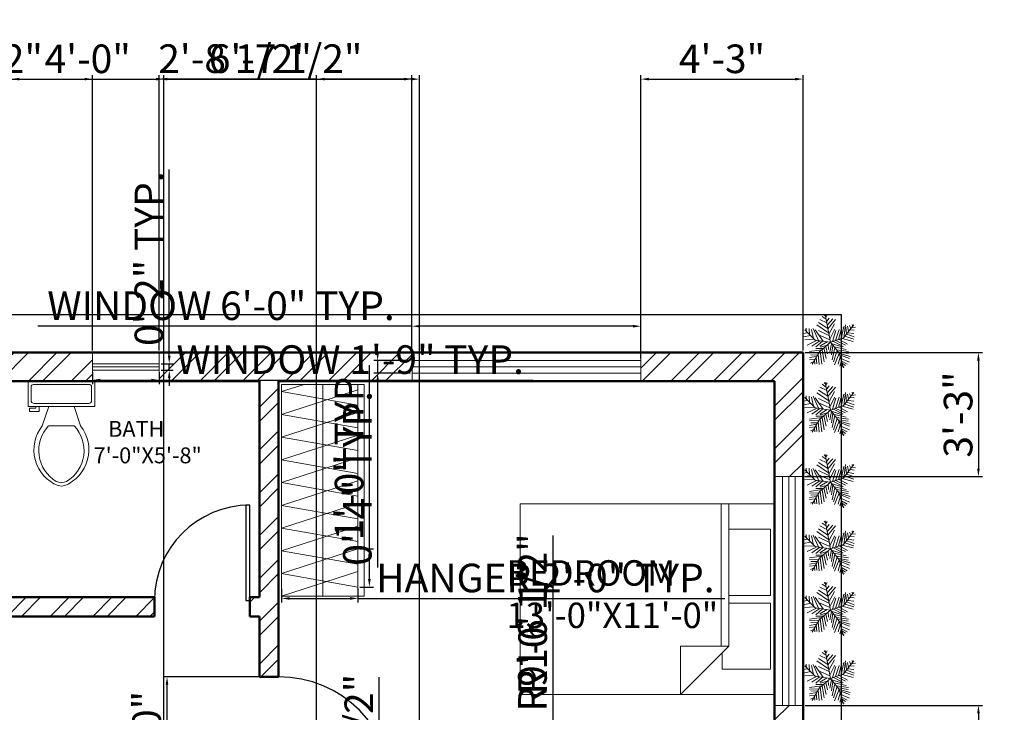
# Model space of a CAD drawing. Units: inches. Extents: x 176 to 806, y 915 to 1663.
# Tile 5 of 5: x 482 to 792, y 1445 to 1663. Entities that reach past the tile are written whole.
import ezdxf

# ---------------------------------------------------------------- set-up
doc = ezdxf.new("R2010")
doc.units = ezdxf.units.IN
for name, color, linetype, lineweight in [('A-ANNO-DIMS', 2, 'Continuous', 18), ('A-AREA-IDEN', 7, 'Continuous', 18), ('A-DOOR', 4, 'Continuous', 25), ('A-FLOR-CASE', 8, 'Continuous', 18), ('A-FLOR-FIXT', 9, 'Continuous', 18), ('A-FURN', 8, 'Continuous', 18), ('A-WALL', 7, 'Continuous', 50), ('A-WALL-PATT', 252, 'Continuous', 13), ('C-PROP', 8, 'Continuous', 25), ('L-PLNT', 3, 'Continuous', 13)]:
    doc.layers.add(name, color=color, linetype=linetype, lineweight=lineweight)
doc.layers.add('A-GLAZ', color=244, linetype='Continuous', lineweight=18, true_color=0x991b1e)
doc.styles.get("Standard").update_dxf_attribs({"font": 'arial.ttf'})
doc.dimstyles.new('ISO-25', dxfattribs={"dimtxt": 9, "dimasz": 2.5, "dimexe": 1.25, "dimexo": 0.625, "dimtad": 1, "dimlunit": 3, "dimtxsty": 'Standard', "dimcen": 2.5, "dimadec": 0, "dimazin": 0, "dimtfac": 1, "dimtmove": 0, "dimatfit": 3, "dimfxl": 1, "dimarcsym": 0})

# ---------------------------------------------------------------- blocks, each defined once
blk = doc.blocks.new('*U3')
for p, q in [((0, 0), (0, -6)), ((-40, 0), (-40, -6))]:
    blk.add_line(p, q)
blk.add_lwpolyline([(0, 0), (0, 40), (-1.75, 40), (-1.75, 0)], close=True)
blk.add_arc((0, 0), 40, 90, 180)
blk = doc.blocks.new('*U8')
for p, q in [((-5.114, 28.097), (-24.676, 40.636)), ((-7.288, 39.707), (-21.778, 46.673)), ((-8.737, 47.138), (-17.069, 52.711)), ((-10.186, 53.64), (-13.084, 55.962)), ((0, 0), (-10.5, 57)), ((-9.099, 51.782), (-6.563, 55.962)), ((-7.65, 43.423), (-2.578, 49.46)), ((-5.839, 35.992), (4.667, 48.067)), ((-5.114, 27.632), (10.463, 46.673)), ((-31.5, 4.5), (-52.5, 25.5)), ((-48.585, 21.131), (-49.309, 29.026)), ((-43.513, 28.561), (-42.427, 15.558)), ((-38.442, 26.239), (-34.819, 7.663)), ((-35.544, 28.097), (-24.314, 3.947)), ((-14.533, 2.09), (-30.834, 25.31)), ((-3.665, 19.273), (-27.574, 35.527)), ((-24.314, 23.917), (-2.941, 13.7)), ((-2.941, 16.486), (8.652, 37.85)), ((-1.129, 6.734), (9.014, 26.704)), ((3.942, 1.625), (11.187, 24.381)), ((10.101, 3.483), (17.708, 26.239)), ((16.259, 5.805), (23.142, 31.348)), ((22.055, 7.198), (27.489, 32.277)), ((27, 9), (48, 36)), ((27.127, 9.056), (31.112, 35.992)), ((31.836, 30.883), (32.561, 16.486)), ((35.096, 32.741), (37.27, 22.524)), ((38.719, 34.134), (41.979, 28.561)), ((40.53, 25.775), (48.862, 24.846)), ((43.791, 29.954), (51.036, 30.883)), ((44.153, 36.456), (45.239, 32.741)), ((-47.498, 19.737), (-55.83, 18.344)), ((-40.615, 13.7), (-55.105, 10.913)), ((-33.37, 6.269), (-52.207, 5.34)), ((-28.299, 3.483), (-47.86, -5.805)), ((-21.416, 3.018), (-38.079, -8.128)), ((0, 0), (-31.5, 4.5)), ((-15.982, 2.09), (-30.11, -9.521)), ((0, 0), (-22.5, -19.5)), ((-6.563, 1.161), (-21.416, -8.128)), ((-20.691, 13.7), (-1.129, 4.876)), ((0, 0), (27, 9)), ((0, 0), (18, -22.5)), ((6.478, 1.625), (26.04, -8.592)), ((11.187, 3.483), (30.749, -5.805)), ((18.07, 5.805), (35.096, -3.483)), ((24.229, 7.663), (46.688, 1.625)), ((29.662, 12.307), (48.137, 6.269)), ((33.285, 16.486), (48.862, 10.913)), ((36.183, 19.737), (48.137, 17.88)), ((-17.431, -15.094), (-42.789, -18.809)), ((-22.5, -19.5), (-37.5, -45)), ((-15.257, -12.772), (-30.11, -12.772)), ((-20.691, -18.345), (-17.793, -44.352)), ((-6.563, -5.805), (-19.967, -9.985)), ((-17.069, -15.094), (-12.721, -40.172)), ((-13.446, -11.378), (-8.737, -32.741)), ((-9.461, -8.592), (-6.201, -23.453)), ((-4.752, -3.483), (-3.665, -14.629)), ((2.493, -3.019), (-1.491, -20.202)), ((1.769, -2.555), (24.229, -9.521)), ((5.029, -6.27), (2.131, -25.775)), ((9.014, -11.378), (3.58, -35.992)), ((14.085, -16.951), (6.478, -40.172)), ((7.565, -9.056), (32.198, -14.629)), ((12.274, -15.094), (36.907, -18.809)), ((16.259, -19.738), (36.183, -22.989)), ((-28.299, -29.026), (-42.789, -31.348)), ((-24.314, -21.596), (-42.427, -22.06)), ((-30.834, -34.135), (-42.427, -35.528)), ((-34.457, -39.708), (-40.978, -42.494)), ((-26.849, -26.24), (-40.253, -25.775)), ((-32.646, -36.921), (-31.921, -44.352)), ((-29.023, -30.884), (-27.936, -43.887)), ((-25.038, -23.918), (-22.865, -45.281)), ((18.07, -22.524), (8.289, -45.745)), ((20.244, -30.419), (15.897, -44.816)), ((18, -22.5), (27, -52.5)), ((18.433, -22.524), (40.53, -29.026)), ((19.157, -25.311), (38.719, -33.206)), ((22.78, -37.85), (19.519, -48.532)), ((21.331, -32.741), (39.081, -40.636)), ((22.78, -38.314), (34.372, -44.816)), ((24.591, -45.745), (23.142, -50.854)), ((24.591, -43.423), (30.749, -47.603)), ((26.764, -49.925), (28.213, -50.854))]:
    blk.add_line(p, q)
blk = doc.blocks.new('Bed - Queen')
for p, q in [((0, -80.00003), (0, 0)), ((0, 0), (59.99999, 0)), ((59.99999, 0), (59.99999, -80.00003)), ((7.99999, -1.2), (28.79998, -1.2)), ((7.99999, -14.4), (7.99999, -1.2)), ((28.79998, -1.2), (28.79998, -14.4)), ((31.19999, -1.2), (51.99999, -1.2)), ((31.19999, -14.4), (31.19999, -1.2)), ((51.99999, -1.2), (51.99999, -16.4)), ((0, -14.4), (44.8, -14.4)), ((59.99999, -29.6), (44.8, -14.4)), ((44.8, -14.4), (44.8, -29.6)), ((44.8, -16.8), (0, -16.8)), ((51.99999, -16.4), (46.79936, -16.4)), ((44.8, -29.6), (59.99999, -29.6)), ((59.99999, -80.00003), (0, -80.00003))]:
    blk.add_line(p, q)
blk = doc.blocks.new('*U13')
for p, q in [((9.5, -6), (9.5, -2)), ((-10, -8.5), (-8, -8.5)), ((-10, -9.5), (-10, -8.5)), ((-8, -8.5), (-8, -8)), ((-7, -8), (-7, -9.5)), ((-4, -8), (-6, -14)), ((4, -8), (6, -14)), ((-7, -9.5), (-10, -9.5)), ((4, -14), (-4, -14))]:
    blk.add_line(p, q)
blk.add_lwpolyline([(10.5, -8), (10.5, 0), (-10.5, 0), (-10.5, -8)], close=True)
for points in [[(-9.5, -2), (-9.5, -6)], [(8.5, -1), (-8.5, -1)], [(-8.5, -7), (8.5, -7)]]:
    blk.add_lwpolyline(points)
for centre, radius, start, end in [((-8.62, -1.88), 0.884, 81.8699, 188.1301), ((8.62, -1.88), 0.884, 351.8699, 98.1301), ((-8.62, -6.12), 0.884, 171.8699, 278.1301), ((8.62, -6.12), 0.884, 261.8699, 8.1301), ((3.52, -21.58), 12.17, 141.4691, 247.9714), ((4.2, -21.82), 11.33, 136.3677, 238.9468), ((-3.52, -21.58), 12.17, 292.0284, 38.5307), ((-4.2, -21.82), 11.33, 301.053, 43.6321), ((0, -27.88), 4, 245.7318, 294.2682), ((0, -29), 4, 254.8605, 285.1395)]:
    blk.add_arc(centre, radius, start, end)
blk = doc.blocks.new('WIN-GLAZING-72IN')
for p, q in [((0, 2), (72, 2)), ((0, 0), (72, 0)), ((0, -2), (72, -2))]:
    blk.add_line(p, q)
blk = doc.blocks.new('WIN-GLAZING-21IN')
for p, q in [((0, 1), (21, 1)), ((0, 0), (21, 0)), ((0, -1), (21, -1))]:
    blk.add_line(p, q)
blk = doc.blocks.new('WARDROBE-HANGER')
for p, q in [((0, 0), (24, 7.76)), ((24, -4.24), (0, 0))]:
    blk.add_line(p, q)
blk = doc.blocks.new('*D22')
at = {"layer": 'A-ANNO-DIMS', "color": 0, "lineweight": -2, "transparency": 16777216}
for p, q in [((564.7, 1483.83), (564.7, 1479.6)), ((588.7, 1483.83), (588.7, 1479.6)), ((567.2, 1480.85), (586.2, 1480.85)), ((588.7, 1480.85), (704.11, 1480.85))]:
    blk.add_line(p, q, dxfattribs=at)
at = {"layer": 'A-ANNO-DIMS', "color": 0, "transparency": 16777216}
for points in [[(567.2, 1481.27), (567.2, 1480.44), (564.7, 1480.85)], [(586.2, 1481.27), (586.2, 1480.44), (588.7, 1480.85)]]:
    blk.add_solid(points, dxfattribs=at)
at = {"layer": 'Defpoints', "color": 0, "transparency": 16777216}
for p in [(564.7, 1484.45), (588.7, 1484.45), (588.7, 1480.85)]:
    blk.add_point(p, dxfattribs=at)
at = {"layer": 'A-ANNO-DIMS', "color": 0, "transparency": 16777216, "insert": (647.66, 1486.13), "char_height": 9, "attachment_point": 5}
blk.add_mtext('HANGER 2\'-0" TYP.', dxfattribs=at)
blk = doc.blocks.new('*D23')
at = {"layer": 'A-ANNO-DIMS', "color": 0, "lineweight": -2, "transparency": 16777216}
for p, q in [((592.3, 1496.45), (592.3, 1554.21)), ((589.33, 1496.45), (593.55, 1496.45)), ((592.3, 1486.95), (592.3, 1493.95)), ((589.33, 1484.45), (593.55, 1484.45))]:
    blk.add_line(p, q, dxfattribs=at)
at = {"layer": 'A-ANNO-DIMS', "color": 0, "transparency": 16777216}
for points in [[(591.89, 1493.95), (592.72, 1493.95), (592.3, 1496.45)], [(591.89, 1486.95), (592.72, 1486.95), (592.3, 1484.45)]]:
    blk.add_solid(points, dxfattribs=at)
at = {"layer": 'Defpoints', "color": 0, "transparency": 16777216}
for p in [(588.7, 1496.45), (592.3, 1496.45), (588.7, 1484.45)]:
    blk.add_point(p, dxfattribs=at)
at = {"layer": 'A-ANNO-DIMS', "color": 0, "transparency": 16777216, "insert": (587.08, 1526.58), "char_height": 9, "attachment_point": 5, "rotation": 90}
blk.add_mtext('1\'-0" TYP.', dxfattribs=at)
blk = doc.blocks.new('*D24')
at = {"layer": 'A-ANNO-DIMS', "color": 0, "lineweight": -2, "transparency": 16777216}
for p, q in [((605.7, 1556.33), (605.7, 1567.76)), ((677.7, 1556.33), (677.7, 1567.76)), ((605.7, 1566.51), (488.07, 1566.51)), ((675.2, 1566.51), (608.2, 1566.51))]:
    blk.add_line(p, q, dxfattribs=at)
at = {"layer": 'A-ANNO-DIMS', "color": 0, "transparency": 16777216}
for points in [[(608.2, 1566.92), (608.2, 1566.09), (605.7, 1566.51)], [(675.2, 1566.92), (675.2, 1566.09), (677.7, 1566.51)]]:
    blk.add_solid(points, dxfattribs=at)
at = {"layer": 'Defpoints', "color": 0, "transparency": 16777216}
for p in [(605.7, 1566.51), (605.7, 1555.71), (677.7, 1555.71)]:
    blk.add_point(p, dxfattribs=at)
at = {"layer": 'A-ANNO-DIMS', "color": 0, "transparency": 16777216, "insert": (545.64, 1571.79), "char_height": 9, "attachment_point": 5}
blk.add_mtext('WINDOW 6\'-0" TYP.', dxfattribs=at)
blk = doc.blocks.new('*D25')
at = {"layer": 'A-ANNO-DIMS', "color": 0, "lineweight": -2, "transparency": 16777216}
for p, q in [((594.9, 1558.21), (594.9, 1560.71)), ((605.08, 1555.71), (593.65, 1555.71)), ((594.9, 1555.71), (594.9, 1551.71)), ((605.08, 1551.71), (593.65, 1551.71)), ((594.9, 1549.21), (594.9, 1490.6))]:
    blk.add_line(p, q, dxfattribs=at)
at = {"layer": 'A-ANNO-DIMS', "color": 0, "transparency": 16777216}
for points in [[(594.49, 1558.21), (595.32, 1558.21), (594.9, 1555.71)], [(594.49, 1549.21), (595.32, 1549.21), (594.9, 1551.71)]]:
    blk.add_solid(points, dxfattribs=at)
at = {"layer": 'Defpoints', "color": 0, "transparency": 16777216}
for p in [(605.7, 1555.71), (594.9, 1551.71), (605.7, 1551.71)]:
    blk.add_point(p, dxfattribs=at)
at = {"layer": 'A-ANNO-DIMS', "color": 0, "transparency": 16777216, "insert": (589.68, 1518.65), "char_height": 9, "attachment_point": 5, "rotation": 90}
blk.add_mtext('0\'-4" TYP.', dxfattribs=at)
blk = doc.blocks.new('*D26')
at = {"layer": 'A-ANNO-DIMS', "color": 0, "lineweight": -2, "transparency": 16777216}
for p, q in [((505.2, 1552.08), (505.2, 1548.31)), ((526.2, 1552.08), (526.2, 1548.31)), ((507.7, 1549.56), (523.7, 1549.56)), ((526.2, 1549.56), (643.84, 1549.56))]:
    blk.add_line(p, q, dxfattribs=at)
at = {"layer": 'A-ANNO-DIMS', "color": 0, "transparency": 16777216}
for points in [[(507.7, 1549.97), (507.7, 1549.14), (505.2, 1549.56)], [(523.7, 1549.97), (523.7, 1549.14), (526.2, 1549.56)]]:
    blk.add_solid(points, dxfattribs=at)
at = {"layer": 'Defpoints', "color": 0, "transparency": 16777216}
for p in [(505.2, 1552.71), (526.2, 1552.71), (526.2, 1549.56)]:
    blk.add_point(p, dxfattribs=at)
at = {"layer": 'A-ANNO-DIMS', "color": 0, "transparency": 16777216, "insert": (586.27, 1554.84), "char_height": 9, "attachment_point": 5}
blk.add_mtext('WINDOW 1\'-9" TYP.', dxfattribs=at)
blk = doc.blocks.new('*D27')
at = {"layer": 'A-ANNO-DIMS', "color": 0, "lineweight": -2, "transparency": 16777216}
for p, q in [((529.35, 1557.21), (529.35, 1615.82)), ((526.83, 1554.71), (530.6, 1554.71)), ((529.35, 1552.71), (529.35, 1554.71)), ((526.83, 1552.71), (530.6, 1552.71)), ((529.35, 1550.21), (529.35, 1547.71))]:
    blk.add_line(p, q, dxfattribs=at)
at = {"layer": 'A-ANNO-DIMS', "color": 0, "transparency": 16777216}
for points in [[(528.94, 1557.21), (529.77, 1557.21), (529.35, 1554.71)], [(528.94, 1550.21), (529.77, 1550.21), (529.35, 1552.71)]]:
    blk.add_solid(points, dxfattribs=at)
at = {"layer": 'Defpoints', "color": 0, "transparency": 16777216}
for p in [(526.2, 1554.71), (529.35, 1554.71), (526.2, 1552.71)]:
    blk.add_point(p, dxfattribs=at)
at = {"layer": 'A-ANNO-DIMS', "color": 0, "transparency": 16777216, "insert": (524.13, 1587.76), "char_height": 9, "attachment_point": 5, "rotation": 90}
blk.add_mtext('0\'-2" TYP.', dxfattribs=at)
blk = doc.blocks.new('*D37')
at = {"layer": 'A-ANNO-DIMS', "color": 0, "lineweight": -2, "transparency": 16777216}
for p, q in [((595.42, 1407.41), (595.42, 1456.05)), ((607.4, 1407.41), (594.17, 1407.41)), ((595.42, 1373.24), (595.42, 1404.91)), ((607.4, 1370.74), (594.17, 1370.74))]:
    blk.add_line(p, q, dxfattribs=at)
at = {"layer": 'A-ANNO-DIMS', "color": 0, "transparency": 16777216}
for points in [[(595.01, 1404.91), (595.84, 1404.91), (595.42, 1407.41)], [(595.01, 1373.24), (595.84, 1373.24), (595.42, 1370.74)]]:
    blk.add_solid(points, dxfattribs=at)
at = {"layer": 'Defpoints', "color": 0, "transparency": 16777216}
for p in [(595.42, 1407.41), (608.02, 1407.41), (608.02, 1370.74)]:
    blk.add_point(p, dxfattribs=at)
at = {"layer": 'A-ANNO-DIMS', "color": 0, "transparency": 16777216, "insert": (590.14, 1432.98), "char_height": 9, "attachment_point": 5, "rotation": 90}
blk.add_mtext('3\'-0 1/2"', dxfattribs=at)
blk = doc.blocks.new('*D41')
at = {"layer": 'A-ANNO-DIMS', "color": 0, "lineweight": -2, "transparency": 16777216}
for p, q in [((425.7, 1558.83), (425.7, 1645.51)), ((505.2, 1558.83), (505.2, 1645.51)), ((428.2, 1644.26), (502.7, 1644.26))]:
    blk.add_line(p, q, dxfattribs=at)
at = {"layer": 'A-ANNO-DIMS', "color": 0, "transparency": 16777216}
for points in [[(428.2, 1644.67), (428.2, 1643.84), (425.7, 1644.26)], [(502.7, 1644.67), (502.7, 1643.84), (505.2, 1644.26)]]:
    blk.add_solid(points, dxfattribs=at)
at = {"layer": 'Defpoints', "color": 0, "transparency": 16777216}
for p in [(505.2, 1644.26), (425.7, 1558.21), (505.2, 1558.21)]:
    blk.add_point(p, dxfattribs=at)
at = {"layer": 'A-ANNO-DIMS', "color": 0, "transparency": 16777216, "insert": (465.45, 1649.53), "char_height": 9, "attachment_point": 5}
blk.add_mtext('6\'-7 1/2"', dxfattribs=at)
blk = doc.blocks.new('*D42')
at = {"layer": 'A-ANNO-DIMS', "color": 0, "lineweight": -2, "transparency": 16777216}
for p, q in [((526.2, 1558.83), (526.2, 1645.51)), ((605.7, 1558.83), (605.7, 1645.51)), ((528.7, 1644.26), (603.2, 1644.26))]:
    blk.add_line(p, q, dxfattribs=at)
at = {"layer": 'A-ANNO-DIMS', "color": 0, "transparency": 16777216}
for points in [[(528.7, 1644.67), (528.7, 1643.84), (526.2, 1644.26)], [(603.2, 1644.67), (603.2, 1643.84), (605.7, 1644.26)]]:
    blk.add_solid(points, dxfattribs=at)
at = {"layer": 'Defpoints', "color": 0, "transparency": 16777216}
for p in [(605.7, 1644.26), (526.2, 1558.21), (605.7, 1558.21)]:
    blk.add_point(p, dxfattribs=at)
at = {"layer": 'A-ANNO-DIMS', "color": 0, "transparency": 16777216, "insert": (565.95, 1649.53), "char_height": 9, "attachment_point": 5}
blk.add_mtext('6\'-7 1/2"', dxfattribs=at)
blk = doc.blocks.new('*D43')
at = {"layer": 'A-ANNO-DIMS', "color": 0, "lineweight": -2, "transparency": 16777216}
for p, q in [((677.7, 1558.83), (677.7, 1645.51)), ((728.7, 1558.83), (728.7, 1645.51)), ((680.2, 1644.26), (726.2, 1644.26))]:
    blk.add_line(p, q, dxfattribs=at)
at = {"layer": 'A-ANNO-DIMS', "color": 0, "transparency": 16777216}
for points in [[(680.2, 1644.67), (680.2, 1643.84), (677.7, 1644.26)], [(726.2, 1644.67), (726.2, 1643.84), (728.7, 1644.26)]]:
    blk.add_solid(points, dxfattribs=at)
at = {"layer": 'Defpoints', "color": 0, "transparency": 16777216}
for p in [(728.7, 1644.26), (677.7, 1558.21), (728.7, 1558.21)]:
    blk.add_point(p, dxfattribs=at)
at = {"layer": 'A-ANNO-DIMS', "color": 0, "transparency": 16777216, "insert": (703.2, 1649.48), "char_height": 9, "attachment_point": 5}
blk.add_mtext('4\'-3"', dxfattribs=at)
blk = doc.blocks.new('*D44')
at = {"layer": 'A-ANNO-DIMS', "color": 0, "lineweight": -2, "transparency": 16777216}
for p, q in [((729.33, 1558.21), (785.1, 1558.21)), ((783.85, 1555.71), (783.85, 1521.71)), ((729.33, 1519.21), (785.1, 1519.21))]:
    blk.add_line(p, q, dxfattribs=at)
at = {"layer": 'A-ANNO-DIMS', "color": 0, "transparency": 16777216}
for points in [[(783.43, 1555.71), (784.27, 1555.71), (783.85, 1558.21)], [(783.43, 1521.71), (784.27, 1521.71), (783.85, 1519.21)]]:
    blk.add_solid(points, dxfattribs=at)
at = {"layer": 'Defpoints', "color": 0, "transparency": 16777216}
for p in [(728.7, 1558.21), (728.7, 1519.21), (783.85, 1519.21)]:
    blk.add_point(p, dxfattribs=at)
at = {"layer": 'A-ANNO-DIMS', "color": 0, "transparency": 16777216, "insert": (778.63, 1538.71), "char_height": 9, "attachment_point": 5, "rotation": 90}
blk.add_mtext('3\'-3"', dxfattribs=at)
blk = doc.blocks.new('*D45')
at = {"layer": 'A-ANNO-DIMS', "color": 0, "lineweight": -2, "transparency": 16777216}
for p, q in [((729.33, 1447.21), (785.1, 1447.21)), ((783.85, 1444.71), (783.85, 1382.17)), ((729.33, 1379.67), (785.1, 1379.67))]:
    blk.add_line(p, q, dxfattribs=at)
at = {"layer": 'A-ANNO-DIMS', "color": 0, "transparency": 16777216}
for points in [[(783.43, 1444.71), (784.27, 1444.71), (783.85, 1447.21)], [(783.43, 1382.17), (784.27, 1382.17), (783.85, 1379.67)]]:
    blk.add_solid(points, dxfattribs=at)
at = {"layer": 'Defpoints', "color": 0, "transparency": 16777216}
for p in [(728.7, 1447.21), (728.7, 1379.67), (783.85, 1379.67)]:
    blk.add_point(p, dxfattribs=at)
at = {"layer": 'A-ANNO-DIMS', "color": 0, "transparency": 16777216, "insert": (778.57, 1413.44), "char_height": 9, "attachment_point": 5, "rotation": 90}
blk.add_mtext('5\'-7 1/2"', dxfattribs=at)
blk = doc.blocks.new('*D52')
at = {"layer": 'A-ANNO-DIMS', "color": 0, "lineweight": -2, "transparency": 16777216}
for p, q in [((479.7, 1200.83), (479.7, 1645.51)), ((527.7, 1200.83), (527.7, 1645.51)), ((482.2, 1644.26), (525.2, 1644.26))]:
    blk.add_line(p, q, dxfattribs=at)
at = {"layer": 'A-ANNO-DIMS', "color": 0, "transparency": 16777216}
for points in [[(482.2, 1644.67), (482.2, 1643.84), (479.7, 1644.26)], [(525.2, 1644.67), (525.2, 1643.84), (527.7, 1644.26)]]:
    blk.add_solid(points, dxfattribs=at)
at = {"layer": 'Defpoints', "color": 0, "transparency": 16777216}
for p in [(527.7, 1644.26), (479.7, 1200.21), (527.7, 1200.21)]:
    blk.add_point(p, dxfattribs=at)
at = {"layer": 'A-ANNO-DIMS', "color": 0, "transparency": 16777216, "insert": (503.7, 1649.48), "char_height": 9, "attachment_point": 5}
blk.add_mtext('4\'-0"', dxfattribs=at)
blk = doc.blocks.new('*D64')
at = {"layer": 'A-ANNO-DIMS', "color": 0, "lineweight": -2, "transparency": 16777216}
for p, q in [((563.08, 1456.21), (527.4, 1456.21)), ((528.65, 1422.71), (528.65, 1453.71)), ((563.08, 1420.21), (527.4, 1420.21))]:
    blk.add_line(p, q, dxfattribs=at)
at = {"layer": 'A-ANNO-DIMS', "color": 0, "transparency": 16777216}
for points in [[(528.24, 1453.71), (529.07, 1453.71), (528.65, 1456.21)], [(528.24, 1422.71), (529.07, 1422.71), (528.65, 1420.21)]]:
    blk.add_solid(points, dxfattribs=at)
at = {"layer": 'Defpoints', "color": 0, "transparency": 16777216}
for p in [(528.65, 1456.21), (563.7, 1456.21), (563.7, 1420.21)]:
    blk.add_point(p, dxfattribs=at)
at = {"layer": 'A-ANNO-DIMS', "color": 0, "transparency": 16777216, "insert": (523.43, 1438.21), "char_height": 9, "attachment_point": 5, "rotation": 90}
blk.add_mtext('3\'-0"', dxfattribs=at)
blk = doc.blocks.new('*D65')
at = {"layer": 'A-ANNO-DIMS', "color": 0, "lineweight": -2, "transparency": 16777216}
for p, q in [((575.7, 1278.83), (575.7, 1645.51)), ((608.02, 1371.37), (608.02, 1645.51)), ((575.7, 1644.26), (526.9, 1644.26)), ((605.52, 1644.26), (578.2, 1644.26))]:
    blk.add_line(p, q, dxfattribs=at)
at = {"layer": 'A-ANNO-DIMS', "color": 0, "transparency": 16777216}
for points in [[(578.2, 1644.67), (578.2, 1643.84), (575.7, 1644.26)], [(605.52, 1644.67), (605.52, 1643.84), (608.02, 1644.26)]]:
    blk.add_solid(points, dxfattribs=at)
at = {"layer": 'Defpoints', "color": 0, "transparency": 16777216}
for p in [(575.7, 1644.26), (608.02, 1370.74), (575.7, 1278.21)]:
    blk.add_point(p, dxfattribs=at)
at = {"layer": 'A-ANNO-DIMS', "color": 0, "transparency": 16777216, "insert": (550.05, 1649.53), "char_height": 9, "attachment_point": 5}
blk.add_mtext('2\'-8 1/2"', dxfattribs=at)
blk = doc.blocks.new('*D74')
at = {"layer": 'A-ANNO-DIMS', "color": 0, "lineweight": -2, "transparency": 16777216}
for p, q in [((650.03, 1491.85), (650.02, 1401.24)), ((650.02, 1277.55), (650.02, 1398.74))]:
    blk.add_line(p, q, dxfattribs=at)
at = {"layer": 'A-ANNO-DIMS', "color": 0, "transparency": 16777216}
blk.add_solid([(649.61, 1401.24), (650.44, 1401.24), (650.02, 1398.74)], dxfattribs=at)
at = {"layer": 'Defpoints', "color": 0, "transparency": 16777216}
for p in [(650.02, 1398.74), (650.02, 1277.55)]:
    blk.add_point(p, dxfattribs=at)
at = {"layer": 'A-ANNO-DIMS', "color": 0, "transparency": 16777216, "insert": (644.81, 1471.46), "char_height": 9, "attachment_point": 5, "rotation": 89.9999}
blk.add_mtext('R10\'-1"', dxfattribs=at)
blk = doc.blocks.new('*D75')
at = {"layer": 'A-ANNO-DIMS', "color": 0, "lineweight": -2, "transparency": 16777216}
for p, q in [((650.03, 1500.67), (650.02, 1407.24)), ((650.02, 1290.49), (650.02, 1404.74))]:
    blk.add_line(p, q, dxfattribs=at)
at = {"layer": 'A-ANNO-DIMS', "color": 0, "transparency": 16777216}
blk.add_solid([(649.61, 1407.24), (650.44, 1407.24), (650.02, 1404.74)], dxfattribs=at)
at = {"layer": 'Defpoints', "color": 0, "transparency": 16777216}
for p in [(650.02, 1404.74), (650.02, 1290.49)]:
    blk.add_point(p, dxfattribs=at)
at = {"layer": 'A-ANNO-DIMS', "color": 0, "transparency": 16777216, "insert": (644.75, 1473.29), "char_height": 9, "attachment_point": 5, "rotation": 89.9998}
blk.add_mtext('R9\'-6 1/2"', dxfattribs=at)

msp = doc.modelspace()

# ---------------------------------------------------------------- hatches: boundary and pattern name
at = {"layer": 'A-WALL-PATT'}
h = msp.add_hatch(dxfattribs=at)
h.set_pattern_fill('ANSI32', color=256)
h.paths.add_polyline_path([(302.704, 1050.206), (353.704, 1050.206), (353.704, 1059.206), (311.704, 1059.206), (311.704, 1191.206), (428.704, 1191.206), (428.704, 1200.206), (311.704, 1200.206), (311.704, 1357.206), (473.704, 1357.206), (473.704, 1363.206), (408.704, 1363.206), (408.704, 1366.206), (402.704, 1366.206), (402.704, 1363.206), (311.704, 1363.206), (311.704, 1376.706), (302.704, 1376.706)])
h.paths.add_polyline_path([(311.704, 1447.206), (302.704, 1447.206), (302.704, 1397.706), (311.704, 1397.706), (311.704, 1411.206), (402.704, 1411.206), (402.704, 1396.206), (408.704, 1396.206), (408.704, 1411.206), (473.704, 1411.206), (473.704, 1420.206), (467.704, 1420.206), (467.704, 1417.206), (311.704, 1417.206)])
h.paths.add_polyline_path([(467.704, 1059.206), (425.704, 1059.206), (425.704, 1050.206), (476.704, 1050.206), (476.704, 1191.206), (479.704, 1191.206), (479.704, 1200.206), (464.704, 1200.206), (464.704, 1191.206), (467.704, 1191.206)])
h.paths.add_polyline_path([(719.704, 1278.206), (614.704, 1278.206), (614.704, 1272.206), (654.704, 1272.206), (654.704, 1250.311), (660.704, 1250.311), (660.704, 1272.206), (719.704, 1272.206), (719.704, 1246.706), (728.704, 1246.706), (728.704, 1307.669), (719.704, 1307.669)])
h.paths.add_polyline_path([(728.704, 1447.206), (719.704, 1447.206), (719.704, 1417.206), (563.704, 1417.206), (563.704, 1420.206), (557.704, 1420.206), (557.704, 1411.206), (569.704, 1411.206), (569.704, 1272.206), (578.704, 1272.206), (578.704, 1278.206), (575.704, 1278.206), (575.704, 1411.206), (719.704, 1411.206), (719.704, 1379.669), (728.704, 1379.669)])
h.paths.add_polyline_path([(677.704, 1558.206), (677.704, 1549.206), (719.704, 1549.206), (719.704, 1519.206), (728.704, 1519.206), (728.704, 1558.206)])
h.paths.add_polyline_path([(526.204, 1558.206), (526.204, 1549.206), (557.704, 1549.206), (557.704, 1481.206), (554.704, 1481.206), (554.704, 1475.206), (557.704, 1475.206), (557.704, 1456.206), (563.704, 1456.206), (563.704, 1549.206), (605.704, 1549.206), (605.704, 1558.206)])
h.paths.add_polyline_path([(425.704, 1558.206), (425.704, 1549.206), (467.704, 1549.206), (467.704, 1456.206), (473.704, 1456.206), (473.704, 1475.206), (524.704, 1475.206), (524.704, 1481.206), (473.704, 1481.206), (473.704, 1549.206), (505.204, 1549.206), (505.204, 1558.206)])
h.paths.add_polyline_path([(311.704, 1549.206), (353.704, 1549.206), (353.704, 1558.206), (302.704, 1558.206), (302.704, 1519.206), (311.704, 1519.206)])

# ---------------------------------------------------------------- linework, layer by layer
at = {"layer": 'A-FLOR-CASE'}
for p, q in [((564.704, 1548.206), (564.704, 1481.534)), ((564.704, 1548.206), (590.704, 1548.206)), ((564.704, 1545.92), (571.777, 1548.206)), ((588.704, 1541.684), (564.704, 1545.92)), ((577.704, 1548.206), (577.704, 1481.534)), ((588.704, 1548.206), (588.704, 1481.534)), ((590.704, 1548.206), (590.704, 1481.534)), ((564.704, 1481.534), (588.704, 1489.293)), ((564.704, 1481.534), (590.704, 1481.534))]:
    msp.add_line(p, q, dxfattribs=at)
at = {"layer": 'A-GLAZ'}
for points in [[(505.204, 1558.206), (526.204, 1558.206), (526.204, 1549.206), (505.204, 1549.206)], [(605.704, 1558.206), (677.704, 1558.206), (677.704, 1549.206), (605.704, 1549.206)], [(728.704, 1519.206), (728.704, 1447.206), (719.704, 1447.206), (719.704, 1519.206)]]:
    msp.add_lwpolyline(points, close=True, dxfattribs=at)
at = {"layer": 'A-WALL'}
for p, q in [((302.704, 1558.206), (728.704, 1558.206)), ((728.704, 1558.206), (728.704, 1050.206)), ((473.704, 1549.206), (557.704, 1549.206)), ((557.704, 1549.206), (557.704, 1481.206)), ((563.704, 1549.206), (563.704, 1456.206)), ((563.704, 1549.206), (719.704, 1549.206)), ((719.704, 1549.206), (719.704, 1417.206)), ((473.704, 1481.206), (524.704, 1481.206)), ((524.704, 1481.206), (524.704, 1475.206)), ((554.704, 1481.206), (554.704, 1475.206)), ((554.704, 1481.206), (557.704, 1481.206)), ((473.704, 1475.206), (524.704, 1475.206)), ((554.704, 1475.206), (557.704, 1475.206)), ((557.704, 1475.206), (557.704, 1456.206)), ((563.704, 1456.206), (557.704, 1456.206))]:
    msp.add_line(p, q, dxfattribs=at)
at = {"layer": 'C-PROP'}
for p, q in [((290.704, 1570.206), (740.704, 1570.206)), ((740.704, 1570.206), (740.704, 1023.206))]:
    msp.add_line(p, q, dxfattribs=at)

# ---------------------------------------------------------------- block references
at = {"layer": 'A-DOOR', "xscale": 0.7500000000000071, "yscale": 0.7500000000000071, "zscale": 0.7500000000000071}
msp.add_blockref('*U3', (554.704, 1480.206), dxfattribs=at)
at = {"layer": 'A-DOOR', "xscale": 0.9, "yscale": 0.9, "zscale": 0.9, "rotation": 269.9999999999985}
msp.add_blockref('*U3', (563.704, 1420.206), dxfattribs=at)
at = {"layer": 'A-FLOR-CASE'}
for p in [(564.704, 1538.766), (564.704, 1531.612), (564.704, 1524.458), (564.704, 1517.304), (564.704, 1510.15), (564.704, 1502.996), (564.704, 1495.842), (564.704, 1488.688)]:
    msp.add_blockref('WARDROBE-HANGER', p, dxfattribs=at)
at = {"layer": 'A-FLOR-FIXT'}
msp.add_blockref('*U13', (495.43, 1549.206), dxfattribs=at)
at = {"layer": 'A-FURN', "rotation": 270}
msp.add_blockref('Bed - Queen', (719.704, 1510.62), dxfattribs=at)
at = {"layer": 'A-GLAZ'}
msp.add_blockref('WIN-GLAZING-21IN', (505.204, 1553.706), dxfattribs=at)
for p, rotation in [((677.704, 1553.706), 180), ((724.204, 1447.206), 90.00000000000003)]:
    msp.add_blockref('WIN-GLAZING-72IN', p, dxfattribs=dict(at, rotation=rotation))
at = {"layer": 'L-PLNT', "xscale": 0.1538165911341002, "yscale": 0.1538165911341002, "zscale": 0.1538165911341002}
for p in [(737.299, 1561.439), (737.299, 1540.127), (737.299, 1517.412), (737.299, 1496.485), (737.299, 1477.215), (737.299, 1455.715)]:
    msp.add_blockref('*U8', p, dxfattribs=at)

# ---------------------------------------------------------------- texts
at = {"layer": 'A-AREA-IDEN', "attachment_point": 1}
for s, width, insert, char_height in [('   BATH\\P7\'-0"X5\'-8"', 33.52633, (505.547, 1536.709), 5), ('BEDROOM\\P13\'-0"X11\'-0"', 67.48766, (635.416, 1492.878), 8)]:
    msp.add_mtext_dynamic_manual_height_columns(s, width=width, gutter_width=12.5, heights=[0], dxfattribs=dict(at, insert=insert, char_height=char_height))

# ---------------------------------------------------------------- dimensions: what is measured, and where the dimension line sits
at = {"layer": 'A-ANNO-DIMS'}
for base, p1, p2, picture, middle in [((505.204, 1644.256), (425.704, 1558.206), (505.204, 1558.206), '*D41', (465.454, 1649.535)), ((605.704, 1644.256), (526.204, 1558.206), (605.704, 1558.206), '*D42', (565.954, 1649.535)), ((575.704, 1644.256), (608.025, 1370.744), (575.704, 1278.206), '*D65', (550.054, 1649.535)), ((527.704, 1644.256), (479.704, 1200.206), (527.704, 1200.206), '*D52', (503.704, 1649.477)), ((728.704, 1644.256), (677.704, 1558.206), (728.704, 1558.206), '*D43', (703.204, 1649.48))]:
    dim = msp.add_linear_dim(base=base, p1=p1, p2=p2, dimstyle='ISO-25', override={"dimdec": 1, "dimlfac": 1, "dimrnd": 0, "dimzin": 1, "dimdsep": 46, "dimlunit": 4, "dimfrac": 2}, dxfattribs=at)
    dim.commit()
    dim.dimension.update_dxf_attribs({"geometry": picture, "text_midpoint": middle})
for base, p1, p2, angle, text, picture, middle in [((529.354, 1554.706), (526.204, 1552.706), (526.204, 1554.706), 90, '<> TYP.', '*D27', (524.134, 1587.761)), ((605.704, 1566.506), (677.704, 1555.706), (605.704, 1555.706), 180, 'WINDOW <> TYP.', '*D24', (545.635, 1571.788)), ((594.904, 1551.706), (605.704, 1555.706), (605.704, 1551.706), 270, '<> TYP.', '*D25', (589.684, 1518.652)), ((592.304, 1496.447), (588.704, 1484.453), (588.704, 1496.447), 90, '<> TYP.', '*D23', (587.084, 1526.578))]:
    dim = msp.add_linear_dim(base=base, p1=p1, p2=p2, angle=angle, text=text, dimstyle='ISO-25', override={"dimdec": 1, "dimlfac": 1, "dimrnd": 0, "dimzin": 1, "dimdsep": 46, "dimlunit": 4, "dimfrac": 2}, dxfattribs=at)
    dim.commit()
    dim.dimension.update_dxf_attribs({"geometry": picture, "text_midpoint": middle})
for base, p1, p2, text, picture, middle in [((526.204, 1549.556), (505.204, 1552.706), (526.204, 1552.706), 'WINDOW <> TYP.', '*D26', (586.273, 1554.838)), ((588.704, 1480.853), (564.704, 1484.453), (588.704, 1484.453), 'HANGER <> TYP.', '*D22', (647.658, 1486.131))]:
    dim = msp.add_linear_dim(base=base, p1=p1, p2=p2, text=text, dimstyle='ISO-25', override={"dimdec": 1, "dimlfac": 1, "dimrnd": 0, "dimzin": 1, "dimdsep": 46, "dimlunit": 4, "dimfrac": 2}, dxfattribs=at)
    dim.commit()
    dim.dimension.update_dxf_attribs({"geometry": picture, "text_midpoint": middle})
for base, p1, p2, picture, middle in [((783.849, 1519.206), (728.704, 1558.206), (728.704, 1519.206), '*D44', (778.626, 1538.706)), ((528.654, 1456.206), (563.704, 1420.206), (563.704, 1456.206), '*D64', (523.431, 1438.206)), ((595.425, 1407.411), (608.025, 1370.744), (608.025, 1407.411), '*D37', (590.143, 1432.981)), ((783.849, 1379.669), (728.704, 1447.206), (728.704, 1379.669), '*D45', (778.571, 1413.438))]:
    dim = msp.add_linear_dim(base=base, p1=p1, p2=p2, angle=90, dimstyle='ISO-25', override={"dimdec": 1, "dimlfac": 1, "dimrnd": 0, "dimzin": 1, "dimdsep": 46, "dimlunit": 4, "dimfrac": 2}, dxfattribs=at)
    dim.commit()
    dim.dimension.update_dxf_attribs({"geometry": picture, "text_midpoint": middle})
for center, mpoint, picture, middle in [((650.024694, 1290.494322), (650.025, 1404.744322), '*D75', (650.0251836, 1473.294322)), ((650.025, 1277.548), (650.025, 1398.744), '*D74', (650.025, 1471.462))]:
    dim = msp.add_radius_dim(center=center, mpoint=mpoint, dimstyle='ISO-25', override={"dimdec": 1, "dimlfac": 1, "dimrnd": 0, "dimzin": 1, "dimdsep": 46, "dimlunit": 4, "dimfrac": 2}, dxfattribs=at)
    dim.commit()
    dim.dimension.update_dxf_attribs({"geometry": picture, "text_midpoint": middle, "dimtype": 164})

doc.saveas('drawing.dxf')
